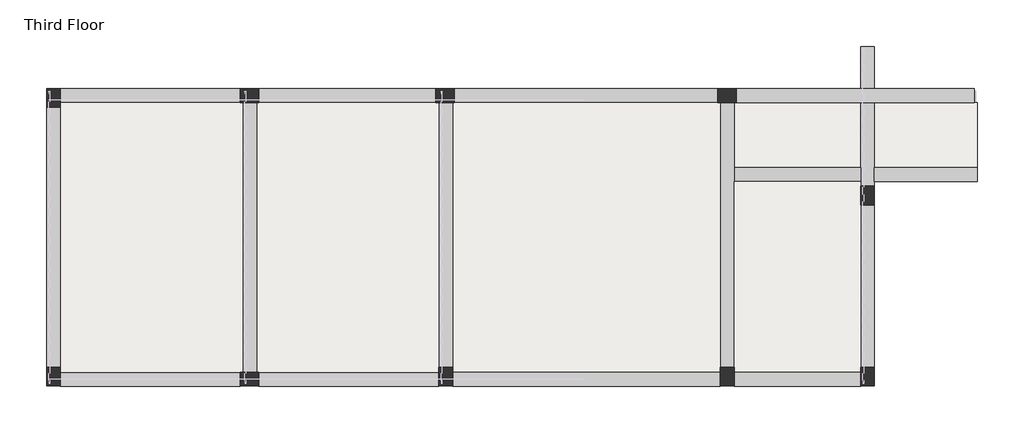
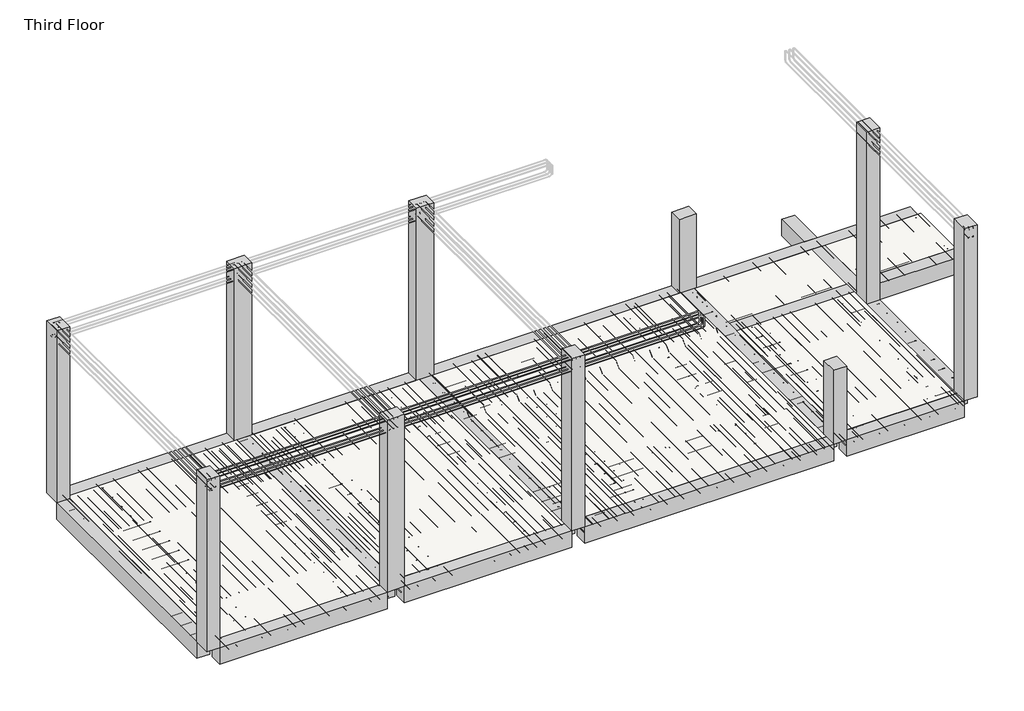
# One storey, part 1 of 4: 10 columns, 8 beams, 5 slabs.
"""IFC4 building model written with IfcOpenShell, lengths in millimetres."""

from ifc_helpers import new_model, si_unit, frame, origin, place, context, project, spatial, polyline, outline, extrude, faceted_brep, element, save

model = new_model("IFC4")

# Units and contexts
model_context = context("Model", 3, world=origin())
ifc_project = project(units=[si_unit("LENGTHUNIT", "METRE", prefix="MILLI")], contexts=[model_context])

# Site, building, storey
site = spatial("IfcSite", under=ifc_project)
building = spatial("IfcBuilding", under=site)
storey = spatial("IfcBuildingStorey", under=building, Name="Third Floor", Elevation=9601.2)

# Beams
placement = place(None, origin())
element("IfcBeam", 1, ObjectType="M_Concrete-Rectangular Beam : 9\" X12\"", at=placement, inside=storey, context=model_context, shape_type="Brep", body=[
    faceted_brep([(3956.0882476, 186.4334631, 9601.2), (3956.0882476, 415.0334631, 9601.2), (1885.9882476, 415.0334631, 9601.2), (1885.9882476, 186.4334631, 9601.2), (3956.0882476, 186.4334631, 9296.4), (1885.9882476, 186.4334631, 9296.4), (3956.0882476, 415.0334631, 9296.4), (1885.9882476, 415.0334631, 9296.4), (3956.0882476, 415.0334631, 9448.8), (1885.9882476, 415.0334631, 9448.8)], [[[0, 1, 2, 3]], [[4, 0, 3, 5]], [[6, 4, 5, 7]], [[1, 8, 6, 7, 9, 2]], [[1, 0, 4, 6, 8]], [[3, 2, 9, 7, 5]]]),
    faceted_brep([(-9150.3117524, 186.4334631, 9601.2), (-9150.3117524, 415.0334631, 9601.2), (-9150.3117524, 415.0334631, 9448.8), (-9150.3117524, 415.0334631, 9296.4), (-9150.3117524, 186.4334631, 9296.4), (-6203.9117524, 415.0334631, 9601.2), (-6203.9117524, 186.4334631, 9601.2), (-6203.9117524, 186.4334631, 9296.4), (-6203.9117524, 415.0334631, 9296.4)], [[[0, 1, 2, 3, 4]], [[5, 6, 7, 8]], [[1, 0, 6, 5]], [[0, 4, 7, 6]], [[4, 3, 8, 7]], [[3, 2, 1, 5, 8]]]),
    faceted_brep([(-5899.1117524, 186.4334631, 9601.2), (-5899.1117524, 415.0334631, 9601.2), (-5899.1117524, 415.0334631, 9296.4), (-5899.1117524, 186.4334631, 9296.4), (-2952.7117524, 415.0334631, 9601.2), (-2952.7117524, 186.4334631, 9601.2), (-2952.7117524, 186.4334631, 9296.4), (-2952.7117524, 415.0334631, 9296.4), (-2952.7117524, 415.0334631, 9448.8)], [[[0, 1, 2, 3]], [[4, 5, 6, 7, 8]], [[1, 0, 5, 4]], [[0, 3, 6, 5]], [[3, 2, 7, 6]], [[2, 1, 4, 8, 7]]]),
    faceted_brep([(-2724.1117524, 186.4334631, 9601.2), (-2724.1117524, 415.0334631, 9601.2), (-2724.1117524, 415.0334631, 9448.8), (-2724.1117524, 415.0334631, 9296.4), (-2724.1117524, 186.4334631, 9296.4), (1657.3882476, 415.0334631, 9601.2), (1657.3882476, 186.4334631, 9601.2), (1657.3882476, 186.4334631, 9296.4), (1657.3882476, 415.0334631, 9296.4), (1657.3882476, 415.0334631, 9448.8)], [[[0, 1, 2, 3, 4]], [[5, 6, 7, 8, 9]], [[1, 0, 6, 5]], [[0, 4, 7, 6]], [[4, 3, 8, 7]], [[3, 2, 1, 5, 9, 8]]]),
])
element("IfcBeam", 2, ObjectType="M_Concrete-Rectangular Beam : 9\" X12\"", at=placement, inside=storey, context=model_context, shape_type="Brep", body=[
    faceted_brep([(3956.0882476, 5755.7334631, 9601.2), (4184.6882476, 5755.7334631, 9601.2), (4184.6882476, 5755.7334631, 9296.4), (3956.0882476, 5755.7334631, 9296.4), (3956.0882476, 5063.2334631, 9601.2), (4184.6882476, 5063.2334631, 9601.2), (4184.6882476, 5063.2334631, 9296.4), (3956.0882476, 5063.2334631, 9296.4)], [[[0, 1, 2, 3]], [[1, 0, 4, 5]], [[2, 1, 5, 6]], [[3, 2, 6, 7]], [[0, 3, 7, 4]], [[5, 4, 7, 6]]]),
    faceted_brep([(4184.6882476, 491.2334631, 9601.2), (3956.0882476, 491.2334631, 9601.2), (3956.0882476, 491.2334631, 9296.4), (4184.6882476, 491.2334631, 9296.4), (3956.0882476, 3158.2334631, 9601.2), (4184.6882476, 3158.2334631, 9601.2), (4184.6882476, 3158.2334631, 9296.4), (3956.0882476, 3158.2334631, 9296.4)], [[[0, 1, 2, 3]], [[4, 5, 6, 7]], [[1, 0, 5, 4]], [[0, 3, 6, 5]], [[3, 2, 7, 6]], [[2, 1, 4, 7]]]),
    faceted_brep([(4184.6882476, 3463.0334631, 9601.2), (3956.0882476, 3463.0334631, 9601.2), (3956.0882476, 3463.0334631, 9296.4), (4184.6882476, 3463.0334631, 9296.4), (3956.0882476, 4834.6334631, 9601.2), (4184.6882476, 4834.6334631, 9601.2), (4184.6882476, 4834.6334631, 9448.8), (4184.6882476, 4834.6334631, 9296.4), (3956.0882476, 4834.6334631, 9296.4), (3956.0882476, 4834.6334631, 9448.8), (4184.6882476, 3539.2334631, 9601.2), (4184.6882476, 3767.8334631, 9601.2), (3956.0882476, 3767.8334631, 9601.2), (3956.0882476, 3539.2334631, 9601.2), (4184.6882476, 3539.2334631, 9296.4), (4184.6882476, 3767.8334631, 9296.4), (3956.0882476, 3539.2334631, 9296.4), (3956.0882476, 3767.8334631, 9296.4)], [[[0, 1, 2, 3]], [[4, 5, 6, 7, 8, 9]], [[1, 0, 10, 11, 5, 4, 12, 13]], [[0, 3, 14, 15, 7, 6, 5, 11, 10]], [[3, 2, 16, 17, 8, 7, 15, 14]], [[2, 1, 13, 12, 4, 9, 8, 17, 16]]]),
])
element("IfcBeam", 3, ObjectType="M_Concrete-Rectangular Beam : 9\" X12\"", at=placement, inside=storey, context=model_context, shape_type="Brep", body=[
    faceted_brep([(5815.3882476, 4834.6334631, 9601.2), (5815.3882476, 4834.6334631, 9296.4), (5815.3882476, 5063.2334631, 9296.4), (5815.3882476, 5063.2334631, 9601.2), (1924.0882476, 4834.6334631, 9601.2), (1924.0882476, 5063.2334631, 9601.2), (1924.0882476, 5063.2334631, 9296.4), (1924.0882476, 4834.6334631, 9296.4), (4184.6882476, 5063.2334631, 9601.2), (3956.0882476, 5063.2334631, 9601.2), (3956.0882476, 4834.6334631, 9601.2), (4184.6882476, 4834.6334631, 9601.2), (4184.6882476, 5063.2334631, 9296.4), (3956.0882476, 5063.2334631, 9296.4), (4184.6882476, 4834.6334631, 9296.4), (3956.0882476, 4834.6334631, 9296.4)], [[[0, 1, 2, 3]], [[4, 5, 6, 7]], [[0, 3, 8, 9, 5, 4, 10, 11]], [[3, 2, 12, 13, 6, 5, 9, 8]], [[2, 1, 14, 15, 7, 6, 13, 12]], [[1, 0, 11, 10, 4, 7, 15, 14]]]),
    faceted_brep([(1619.2882476, 4834.6334631, 9601.2), (1619.2882476, 5063.2334631, 9601.2), (-2698.7117524, 5063.2334631, 9601.2), (-2698.7117524, 4834.6334631, 9601.2), (1619.2882476, 5063.2334631, 9296.4), (-2698.7117524, 5063.2334631, 9296.4), (1619.2882476, 4834.6334631, 9296.4), (-2698.7117524, 4834.6334631, 9296.4)], [[[0, 1, 2, 3]], [[1, 4, 5, 2]], [[4, 6, 7, 5]], [[6, 0, 3, 7]], [[1, 0, 6, 4]], [[2, 5, 7, 3]]]),
    faceted_brep([(-9150.3117524, 4834.6334631, 9601.2), (-9150.3117524, 5063.2334631, 9601.2), (-9150.3117524, 5063.2334631, 9296.4), (-9150.3117524, 4834.6334631, 9296.4), (-9150.3117524, 4834.6334631, 9448.8), (-6203.9117524, 5063.2334631, 9601.2), (-6203.9117524, 5063.2334631, 9296.4), (-6203.9117524, 4834.6334631, 9601.2), (-6203.9117524, 4834.6334631, 9296.4)], [[[0, 1, 2, 3, 4]], [[2, 1, 5, 6]], [[6, 5, 7, 8]], [[1, 0, 7, 5]], [[3, 2, 6, 8]], [[0, 4, 3, 8, 7]]]),
    faceted_brep([(-3003.5117524, 5063.2334631, 9296.4), (-3003.5117524, 5063.2334631, 9601.2), (-3003.5117524, 4834.6334631, 9601.2), (-3003.5117524, 4834.6334631, 9296.4), (-5899.1117524, 5063.2334631, 9601.2), (-5899.1117524, 5063.2334631, 9296.4), (-5899.1117524, 4834.6334631, 9296.4), (-5899.1117524, 4834.6334631, 9601.2)], [[[0, 1, 2, 3]], [[4, 5, 6, 7]], [[1, 0, 5, 4]], [[2, 1, 4, 7]], [[0, 3, 6, 5]], [[3, 2, 7, 6]]]),
])
element("IfcBeam", 4, ObjectType="M_Concrete-Rectangular Beam : 9\" X12\"", at=placement, inside=storey, context=model_context, shape_type="SweptSolid", body=[
    extrude(outline(polyline([(-9378.9117524, 4758.4334631), (-9150.3117524, 4758.4334631), (-9150.3117524, 491.2334631), (-9378.9117524, 491.2334631), (-9378.9117524, 4758.4334631)])), frame((0.0, 0.0, 9296.4), z_axis=(0.0, 0.0, 1.0), x_axis=(1.0, 0.0, 0.0)), (0.0, 0.0, 1.0), 304.8),
])
element("IfcBeam", 5, ObjectType="M_Concrete-Rectangular Beam : 9\" X12\"", at=placement, inside=storey, context=model_context, shape_type="Brep", body=[
    faceted_brep([(-6165.8117524, 415.0334631, 9601.2), (-5937.2117524, 415.0334631, 9601.2), (-5937.2117524, 4834.6334631, 9601.2), (-6165.8117524, 4834.6334631, 9601.2), (-5937.2117524, 415.0334631, 9448.8), (-5937.2117524, 415.0334631, 9296.4), (-5937.2117524, 4834.6334631, 9296.4), (-5937.2117524, 4834.6334631, 9448.8), (-6165.8117524, 415.0334631, 9296.4), (-6165.8117524, 4834.6334631, 9296.4), (-6165.8117524, 415.0334631, 9448.8), (-6165.8117524, 4834.6334631, 9448.8)], [[[0, 1, 2, 3]], [[1, 4, 5, 6, 7, 2]], [[5, 8, 9, 6]], [[8, 10, 0, 3, 11, 9]], [[1, 0, 10, 8, 5, 4]], [[3, 2, 7, 6, 9, 11]]]),
])
element("IfcBeam", 6, ObjectType="M_Concrete-Rectangular Beam : 9\" X12\"", at=placement, inside=storey, context=model_context, shape_type="Brep", body=[
    faceted_brep([(-2952.7117524, 491.2334631, 9601.2), (-2724.1117524, 491.2334631, 9601.2), (-2724.1117524, 4834.6334631, 9601.2), (-2952.7117524, 4834.6334631, 9601.2), (-2724.1117524, 491.2334631, 9296.4), (-2724.1117524, 4834.6334631, 9296.4), (-2724.1117524, 4834.6334631, 9448.8), (-2952.7117524, 491.2334631, 9296.4), (-2952.7117524, 4834.6334631, 9296.4), (-2952.7117524, 4834.6334631, 9448.8)], [[[0, 1, 2, 3]], [[1, 4, 5, 6, 2]], [[4, 7, 8, 5]], [[7, 0, 3, 9, 8]], [[1, 0, 7, 4]], [[3, 2, 6, 5, 8, 9]]]),
])
element("IfcBeam", 7, ObjectType="M_Concrete-Rectangular Beam : 9\" X12\"", at=placement, inside=storey, context=model_context, shape_type="Brep", body=[
    faceted_brep([(1657.3882476, 491.2334631, 9601.2), (1885.9882476, 491.2334631, 9601.2), (1885.9882476, 3539.2334631, 9601.2), (1885.9882476, 3767.8334631, 9601.2), (1885.9882476, 4834.6334631, 9601.2), (1657.3882476, 4834.6334631, 9601.2), (1885.9882476, 491.2334631, 9296.4), (1885.9882476, 3539.2334631, 9296.4), (1885.9882476, 3767.8334631, 9296.4), (1885.9882476, 4834.6334631, 9296.4), (1885.9882476, 4834.6334631, 9448.8), (1657.3882476, 491.2334631, 9296.4), (1657.3882476, 4834.6334631, 9296.4), (1657.3882476, 4834.6334631, 9448.8)], [[[0, 1, 2, 3, 4, 5]], [[1, 6, 7, 8, 9, 10, 4, 3, 2]], [[6, 11, 12, 9, 8, 7]], [[11, 0, 5, 13, 12]], [[1, 0, 11, 6]], [[5, 4, 10, 9, 12, 13]]]),
])
element("IfcBeam", 8, ObjectType="M_Concrete-Rectangular Beam : 9\" X12\"", at=placement, inside=storey, context=model_context, shape_type="Brep", body=[
    faceted_brep([(5871.6882476, 3539.2334631, 9601.2), (5871.6882476, 3539.2334631, 9296.4), (5871.6882476, 3767.8334631, 9296.4), (5871.6882476, 3767.8334631, 9448.8), (5871.6882476, 3767.8334631, 9601.2), (4184.6882476, 3539.2334631, 9601.2), (4184.6882476, 3767.8334631, 9601.2), (4184.6882476, 3767.8334631, 9448.8), (4184.6882476, 3767.8334631, 9296.4), (4184.6882476, 3539.2334631, 9296.4)], [[[0, 1, 2, 3, 4]], [[5, 6, 7, 8, 9]], [[0, 4, 6, 5]], [[4, 3, 2, 8, 7, 6]], [[2, 1, 9, 8]], [[1, 0, 5, 9]]]),
    faceted_brep([(1885.9882476, 3767.8334631, 9601.2), (1885.9882476, 3539.2334631, 9601.2), (3956.0882476, 3539.2334631, 9601.2), (3956.0882476, 3767.8334631, 9601.2), (1885.9882476, 3767.8334631, 9296.4), (1885.9882476, 3767.8334631, 9448.8), (3956.0882476, 3767.8334631, 9448.8), (3956.0882476, 3767.8334631, 9296.4), (1885.9882476, 3539.2334631, 9296.4), (3956.0882476, 3539.2334631, 9296.4), (1885.9882476, 3539.2334631, 9448.8), (3956.0882476, 3539.2334631, 9448.8)], [[[0, 1, 2, 3]], [[4, 5, 0, 3, 6, 7]], [[8, 4, 7, 9]], [[1, 10, 8, 9, 11, 2]], [[1, 0, 5, 4, 8, 10]], [[3, 2, 11, 9, 7, 6]]]),
])

# Columns
element("IfcColumn", 9, ObjectType="M_Concrete-Rectangular-Column : 9\" x 12\"", at=placement, inside=storey, context=model_context, shape_type="SweptSolid", body=[
    extrude(outline(polyline([(-9150.3117524, 5063.2334631), (-9150.3117524, 4758.4334631), (-9378.9117524, 4758.4334631), (-9378.9117524, 5063.2334631), (-9150.3117524, 5063.2334631)])), frame((0.0, 0.0, 9601.2), z_axis=(0.0, 0.0, 1.0), x_axis=(1.0, 0.0, 0.0)), (0.0, 0.0, 1.0), 3200.4),
])
element("IfcColumn", 10, ObjectType="M_Concrete-Rectangular-Column : 9\" x 12\"", at=placement, inside=storey, context=model_context, shape_type="SweptSolid", body=[
    extrude(outline(polyline([(-9150.3117524, 491.2334631), (-9150.3117524, 186.4334631), (-9378.9117524, 186.4334631), (-9378.9117524, 491.2334631), (-9150.3117524, 491.2334631)])), frame((0.0, 0.0, 9601.2), z_axis=(0.0, 0.0, 1.0), x_axis=(1.0, 0.0, 0.0)), (0.0, 0.0, 1.0), 3200.4),
])
element("IfcColumn", 11, ObjectType="M_Concrete-Rectangular-Column : 9\" x 12\"", at=placement, inside=storey, context=model_context, shape_type="Brep", body=[
    faceted_brep([(-6203.9117524, 415.0334631, 9601.2), (-5899.1117524, 415.0334631, 9601.2), (-5899.1117524, 186.4334631, 9601.2), (-6203.9117524, 186.4334631, 9601.2), (-6203.9117524, 415.0334631, 12801.6), (-5899.1117524, 415.0334631, 12801.6), (-5899.1117524, 415.0334631, 12496.8), (-6203.9117524, 415.0334631, 12496.8), (-5899.1117524, 186.4334631, 12801.6), (-5899.1117524, 186.4334631, 12496.8), (-6203.9117524, 186.4334631, 12801.6), (-6203.9117524, 186.4334631, 12496.8)], [[[0, 1, 2, 3]], [[4, 5, 6, 1, 0, 7]], [[5, 8, 9, 2, 1, 6]], [[8, 10, 11, 3, 2, 9]], [[10, 4, 7, 0, 3, 11]], [[4, 10, 8, 5]]]),
])
element("IfcColumn", 12, ObjectType="M_Concrete-Rectangular-Column : 9\" x 12\"", at=placement, inside=storey, context=model_context, shape_type="Brep", body=[
    faceted_brep([(-2952.7117524, 186.4334631, 9601.2), (-2952.7117524, 491.2334631, 9601.2), (-2724.1117524, 491.2334631, 9601.2), (-2724.1117524, 186.4334631, 9601.2), (-2952.7117524, 186.4334631, 12801.6), (-2952.7117524, 415.0334631, 12801.6), (-2952.7117524, 491.2334631, 12801.6), (-2952.7117524, 186.4334631, 12496.8), (-2724.1117524, 491.2334631, 12801.6), (-2724.1117524, 415.0334631, 12801.6), (-2724.1117524, 186.4334631, 12801.6), (-2724.1117524, 186.4334631, 12496.8)], [[[0, 1, 2, 3]], [[4, 5, 6, 1, 0, 7]], [[6, 8, 2, 1]], [[8, 9, 10, 11, 3, 2]], [[10, 4, 7, 0, 3, 11]], [[4, 10, 9, 8, 6, 5]]]),
])
element("IfcColumn", 13, ObjectType="M_Concrete-Rectangular-Column : 9\" x 12\"", at=placement, inside=storey, context=model_context, shape_type="SweptSolid", body=[
    extrude(outline(polyline([(1657.3882476, 186.4334631), (1657.3882476, 491.2334631), (1885.9882476, 491.2334631), (1885.9882476, 186.4334631), (1657.3882476, 186.4334631)])), frame((0.0, 0.0, 9601.2), z_axis=(0.0, 0.0, 1.0), x_axis=(1.0, 0.0, 0.0)), (0.0, 0.0, 1.0), 1371.6),
])
element("IfcColumn", 14, ObjectType="M_Concrete-Rectangular-Column : 9\" x 12\"", at=placement, inside=storey, context=model_context, shape_type="SweptSolid", body=[
    extrude(outline(polyline([(3956.0882476, 186.4334631), (3956.0882476, 491.2334631), (4184.6882476, 491.2334631), (4184.6882476, 186.4334631), (3956.0882476, 186.4334631)])), frame((0.0, 0.0, 9601.2), z_axis=(0.0, 0.0, 1.0), x_axis=(1.0, 0.0, 0.0)), (0.0, 0.0, 1.0), 3200.4),
])
element("IfcColumn", 15, ObjectType="M_Concrete-Rectangular-Column : 9\" x 12\"", at=placement, inside=storey, context=model_context, shape_type="Brep", body=[
    faceted_brep([(3956.0882476, 3158.2334631, 9601.2), (3956.0882476, 3463.0334631, 9601.2), (4184.6882476, 3463.0334631, 9601.2), (4184.6882476, 3158.2334631, 9601.2), (3956.0882476, 3158.2334631, 12801.6), (3956.0882476, 3463.0334631, 12801.6), (3956.0882476, 3463.0334631, 12496.8), (3956.0882476, 3158.2334631, 12496.8), (4184.6882476, 3463.0334631, 12801.6), (4184.6882476, 3463.0334631, 12496.8), (4184.6882476, 3158.2334631, 12801.6), (4184.6882476, 3158.2334631, 12496.8)], [[[0, 1, 2, 3]], [[4, 5, 6, 1, 0, 7]], [[5, 8, 9, 2, 1, 6]], [[8, 10, 11, 3, 2, 9]], [[10, 4, 7, 0, 3, 11]], [[4, 10, 8, 5]]]),
])
element("IfcColumn", 16, ObjectType="M_Concrete-Rectangular-Column : 9\" x 12\"", at=placement, inside=storey, context=model_context, shape_type="SweptSolid", body=[
    extrude(outline(polyline([(1924.0882476, 4834.6334631), (1619.2882476, 4834.6334631), (1619.2882476, 5063.2334631), (1924.0882476, 5063.2334631), (1924.0882476, 4834.6334631)])), frame((0.0, 0.0, 9601.2), z_axis=(0.0, 0.0, 1.0), x_axis=(1.0, 0.0, 0.0)), (0.0, 0.0, 1.0), 1371.6),
])
element("IfcColumn", 17, ObjectType="M_Concrete-Rectangular-Column : 9\" x 12\"", at=placement, inside=storey, context=model_context, shape_type="Brep", body=[
    faceted_brep([(-2698.7117524, 4834.6334631, 9601.2), (-3003.5117524, 4834.6334631, 9601.2), (-3003.5117524, 5063.2334631, 9601.2), (-2698.7117524, 5063.2334631, 9601.2), (-2698.7117524, 4834.6334631, 12801.6), (-3003.5117524, 4834.6334631, 12801.6), (-3003.5117524, 4834.6334631, 12496.8), (-2698.7117524, 4834.6334631, 12496.8), (-3003.5117524, 5063.2334631, 12801.6), (-3003.5117524, 5063.2334631, 12496.8), (-2698.7117524, 5063.2334631, 12801.6), (-2698.7117524, 5063.2334631, 12496.8)], [[[0, 1, 2, 3]], [[4, 5, 6, 1, 0, 7]], [[5, 8, 9, 2, 1, 6]], [[8, 10, 11, 3, 2, 9]], [[10, 4, 7, 0, 3, 11]], [[4, 10, 8, 5]]]),
])
element("IfcColumn", 18, ObjectType="M_Concrete-Rectangular-Column : 9\" x 12\"", at=placement, inside=storey, context=model_context, shape_type="Brep", body=[
    faceted_brep([(-5899.1117524, 4834.6334631, 9601.2), (-6203.9117524, 4834.6334631, 9601.2), (-6203.9117524, 5063.2334631, 9601.2), (-5899.1117524, 5063.2334631, 9601.2), (-5899.1117524, 4834.6334631, 12801.6), (-6203.9117524, 4834.6334631, 12801.6), (-6203.9117524, 4834.6334631, 12496.8), (-5899.1117524, 4834.6334631, 12496.8), (-6203.9117524, 5063.2334631, 12801.6), (-6203.9117524, 5063.2334631, 12496.8), (-5899.1117524, 5063.2334631, 12801.6), (-5899.1117524, 5063.2334631, 12496.8)], [[[0, 1, 2, 3]], [[4, 5, 6, 1, 0, 7]], [[5, 8, 9, 2, 1, 6]], [[8, 10, 11, 3, 2, 9]], [[10, 4, 7, 0, 3, 11]], [[4, 10, 8, 5]]]),
])

# Slabs
element("IfcSlab", 19, ObjectType="FLOOR SLAB 6\"", at=placement, inside=storey, context=model_context, shape_type="Brep", body=[
    faceted_brep([(-6165.8117524, 4834.6334631, 9448.8), (-6165.8117524, 415.0334631, 9448.8), (-9150.3117524, 415.0334631, 9448.8), (-9150.3117524, 4834.6334631, 9448.8), (-6165.8117524, 4834.6334631, 9601.2), (-6203.9117524, 4834.6334631, 9601.2), (-9150.3117524, 4834.6334631, 9601.2), (-9150.3117524, 4758.4334631, 9601.2), (-9150.3117524, 491.2334631, 9601.2), (-9150.3117524, 415.0334631, 9601.2), (-6203.9117524, 415.0334631, 9601.2), (-6165.8117524, 415.0334631, 9601.2)], [[[0, 1, 2, 3]], [[4, 5, 6, 7, 8, 9, 10, 11]], [[1, 0, 4, 11]], [[2, 1, 11, 10, 9]], [[3, 2, 9, 8, 7, 6]], [[0, 3, 6, 5, 4]]]),
])
element("IfcSlab", 20, ObjectType="FLOOR SLAB 6\"", at=placement, inside=storey, context=model_context, shape_type="Brep", body=[
    faceted_brep([(-2952.7117524, 4834.6334631, 9448.8), (-2952.7117524, 415.0334631, 9448.8), (-5937.2117524, 415.0334631, 9448.8), (-5937.2117524, 4834.6334631, 9448.8), (-2952.7117524, 4834.6334631, 9601.2), (-3003.5117524, 4834.6334631, 9601.2), (-5899.1117524, 4834.6334631, 9601.2), (-5937.2117524, 4834.6334631, 9601.2), (-5937.2117524, 415.0334631, 9601.2), (-5899.1117524, 415.0334631, 9601.2), (-2952.7117524, 415.0334631, 9601.2), (-2952.7117524, 491.2334631, 9601.2)], [[[0, 1, 2, 3]], [[4, 5, 6, 7, 8, 9, 10, 11]], [[1, 0, 4, 11, 10]], [[2, 1, 10, 9, 8]], [[3, 2, 8, 7]], [[0, 3, 7, 6, 5, 4]]]),
])
element("IfcSlab", 21, ObjectType="FLOOR SLAB 6\"", at=placement, inside=storey, context=model_context, shape_type="Brep", body=[
    faceted_brep([(1657.3882476, 4834.6334631, 9448.8), (1657.3882476, 415.0334631, 9448.8), (-2724.1117524, 415.0334631, 9448.8), (-2724.1117524, 4834.6334631, 9448.8), (1657.3882476, 4834.6334631, 9601.2), (1619.2882476, 4834.6334631, 9601.2), (-2698.7117524, 4834.6334631, 9601.2), (-2724.1117524, 4834.6334631, 9601.2), (-2724.1117524, 491.2334631, 9601.2), (-2724.1117524, 415.0334631, 9601.2), (1657.3882476, 415.0334631, 9601.2), (1657.3882476, 491.2334631, 9601.2)], [[[0, 1, 2, 3]], [[4, 5, 6, 7, 8, 9, 10, 11]], [[1, 0, 4, 11, 10]], [[2, 1, 10, 9]], [[3, 2, 9, 8, 7]], [[0, 3, 7, 6, 5, 4]]]),
])
element("IfcSlab", 22, ObjectType="FLOOR SLAB 6\"", at=placement, inside=storey, context=model_context, shape_type="Brep", body=[
    faceted_brep([(3956.0882476, 415.0334631, 9448.8), (1885.9882476, 415.0334631, 9448.8), (1885.9882476, 3539.2334631, 9448.8), (3956.0882476, 3539.2334631, 9448.8), (3956.0882476, 415.0334631, 9601.2), (3956.0882476, 491.2334631, 9601.2), (3956.0882476, 3158.2334631, 9601.2), (3956.0882476, 3463.0334631, 9601.2), (3956.0882476, 3539.2334631, 9601.2), (1885.9882476, 3539.2334631, 9601.2), (1885.9882476, 491.2334631, 9601.2), (1885.9882476, 415.0334631, 9601.2)], [[[0, 1, 2, 3]], [[4, 5, 6, 7, 8, 9, 10, 11]], [[1, 0, 4, 11]], [[2, 1, 11, 10, 9]], [[3, 2, 9, 8]], [[0, 3, 8, 7, 6, 5, 4]]]),
])
element("IfcSlab", 23, ObjectType="FLOOR SLAB 6\"", at=placement, inside=storey, context=model_context, shape_type="Brep", body=[
    faceted_brep([(3956.0882476, 3767.8334631, 9448.8), (1885.9882476, 3767.8334631, 9448.8), (1885.9882476, 4834.6334631, 9448.8), (3956.0882476, 4834.6334631, 9448.8), (3956.0882476, 3767.8334631, 9601.2), (3956.0882476, 4834.6334631, 9601.2), (1924.0882476, 4834.6334631, 9601.2), (1885.9882476, 4834.6334631, 9601.2), (1885.9882476, 3767.8334631, 9601.2)], [[[0, 1, 2, 3]], [[4, 5, 6, 7, 8]], [[1, 0, 4, 8]], [[2, 1, 8, 7]], [[3, 2, 7, 6, 5]], [[0, 3, 5, 4]]]),
    faceted_brep([(5871.6882476, 4834.6334631, 9448.8), (5871.6882476, 3767.8334631, 9448.8), (4184.6882476, 3767.8334631, 9448.8), (4184.6882476, 4834.6334631, 9448.8), (5871.6882476, 4834.6334631, 9601.2), (5815.3882476, 4834.6334631, 9601.2), (4184.6882476, 4834.6334631, 9601.2), (4184.6882476, 3767.8334631, 9601.2), (5871.6882476, 3767.8334631, 9601.2)], [[[0, 1, 2, 3]], [[4, 5, 6, 7, 8]], [[1, 0, 4, 8]], [[2, 1, 8, 7]], [[3, 2, 7, 6]], [[0, 3, 6, 5, 4]]]),
])

save(model, "model.ifc")

# Revit data of these elements
# Type "M_Concrete-Rectangular Beam : 9\" X12\""
#   Length [instance default] = 5' - 0"
#   b = 0' - 9"
#   h = 1' - 0"
#   Structural Material [instance default] = Concrete, Cast-in-Place gray
#   Assembly Code = ""
# Type "M_Concrete-Rectangular-Column : 9\" x 12\""
#   b = 0' - 9"
#   h = 1' - 0"
#   Structural Material [instance default] = Concrete, Cast-in-Place gray
# Type "FLOOR SLAB 6\""
#   Layers, outside or top first: 0' - 6" "Concrete, Cast-in-Place gray" (function 1)
# Elements 1, 2, 3, 4, 5, 6, 7, 8 (IfcBeam, "M_Concrete-Rectangular Beam : 9\" X12\"")
#   Structural Material = Concrete, Cast-in-Place gray
#   Phase Created = New Construction
#   Materials on its faces: "Concrete, Cast-in-Place gray"
# Elements 9, 10, 11, 12, 13, 14, 15, 16, 17, 18 (IfcColumn, "M_Concrete-Rectangular-Column : 9\" x 12\"")
#   Structural Material = Concrete, Cast-in-Place gray
#   Phase Created = New Construction
#   Materials on its faces: "Concrete, Cast-in-Place gray"
# Elements 19, 20, 21, 22, 23 (IfcSlab, "FLOOR SLAB 6\"")
#   Height Offset From Level = 0' - 0"
#   built-in parameter 1001954 = 1
#   Phase Created = New Construction
#   Materials on its faces: "Concrete, Cast-in-Place gray"
# Materials
#   "Concrete, Cast-in-Place gray": class "Concrete", colour RGB 192 192 192, transparency 0, Description = "Cast-in-place concrete", Cost = 0
